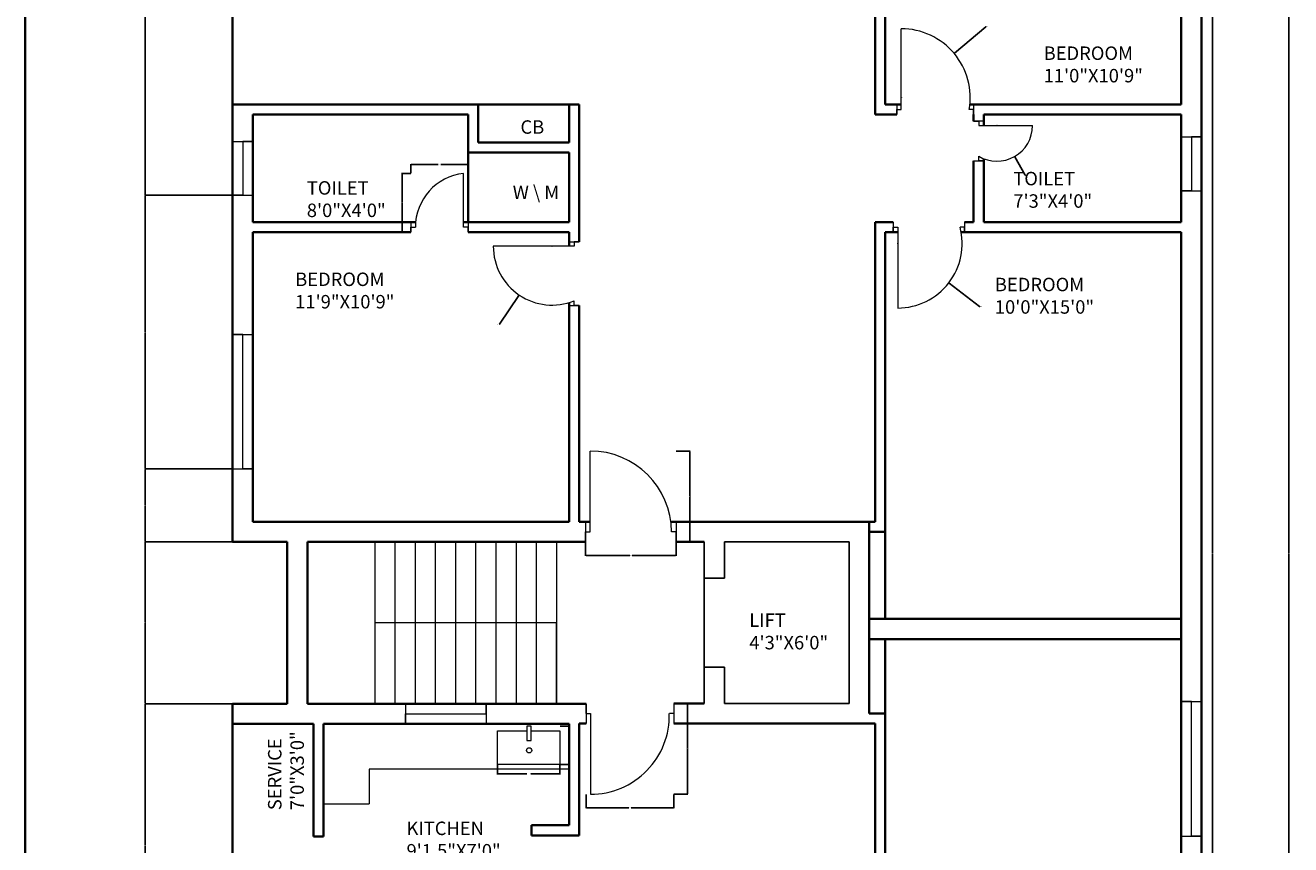
# Model space of a CAD drawing. Units: inches. Extents: x 2250 to 3547, y 1387 to 2604.
# Tile 2 of 11: x 2250 to 2814, y 1765 to 2130. Entities that reach past the tile are written whole.
import ezdxf

# ---------------------------------------------------------------- set-up
doc = ezdxf.new("R2010")
doc.units = ezdxf.units.IN
for name, color, linetype, lineweight in [('A-ANNO-DIMS', 2, 'Continuous', 18), ('A-ANNO-TTLB', 7, 'Continuous', 35), ('A-AREA-IDEN', 7, 'Continuous', 18), ('A-DOOR', 3, 'Continuous', 18), ('A-FLOR-CASE', 9, 'Continuous', 18), ('A-FLOR-EVTR', 6, 'Continuous', 25), ('A-FLOR-FIXT', 8, 'Continuous', 18), ('A-FLOR-STRS', 7, 'Continuous', 18), ('A-GLAZ', 4, 'Continuous', 18), ('A-WALL', 7, 'Continuous', 35)]:
    doc.layers.add(name, color=color, linetype=linetype, lineweight=lineweight)
doc.styles.get("Standard").update_dxf_attribs({"font": 'arial.ttf'})
doc.dimstyles.get("Standard").update_dxf_attribs({"dimtxt": 0.18, "dimasz": 0.18, "dimexe": 0.18, "dimexo": 0.0625, "dimgap": 0.09, "dimtad": 0, "dimtih": 1, "dimtoh": 1, "dimdec": 4, "dimzin": 0, "dimdsep": 46, "dimtxsty": 'Standard', "dimcen": 0.09, "dimadec": 0, "dimazin": 0, "dimtfac": 1, "dimtdec": 4, "dimtofl": 0, "dimtmove": 0, "dimatfit": 3, "dimfxl": 1, "dimtolj": 1, "dimtzin": 0, "dimarcsym": 0})

# ---------------------------------------------------------------- blocks, each defined once
blk = doc.blocks.new('WIN-24')
for p, q in [((0, 24), (9, 24)), ((9, 24), (4.5, 24)), ((4.5, 24), (4.5, 0)), ((4.5, 0), (0, 0)), ((0, 0), (9, 0))]:
    blk.add_line(p, q)
blk = doc.blocks.new('WIN-60')
for p, q in [((0, 9), (0, 0)), ((60, 4.5), (60, 9)), ((60, 9), (60, 0)), ((0, 0), (0, 4.5)), ((0, 4.5), (60, 4.5))]:
    blk.add_line(p, q)
blk = doc.blocks.new('WIN-36')
for p, q in [((0, 9), (0, 0)), ((36, 4.5), (36, 9)), ((36, 9), (36, 0)), ((0, 0), (0, 4.5)), ((0, 4.5), (36, 4.5))]:
    blk.add_line(p, q)
blk = doc.blocks.new('DOOR-BED-NORTHEAST')
for p, q in [((2, 2.25), (2, 38.25)), ((0, 4.5), (0, 0)), ((0, 0), (0, 2.25)), ((0, 2.25), (2, 2.25)), ((34.25, 2.25), (32.25, 2.25)), ((34.25, 4.5), (34.25, 0)), ((34.25, 0), (34.25, 2.25))]:
    blk.add_line(p, q)
blk.add_arc((2, 7.54), 30.71, 350.0755, 90)
blk = doc.blocks.new('DOOR-BED-WEST-N')
for p, q in [((33.75, 28.33), (38.25, 28.33)), ((38.25, 28.33), (36, 28.33)), ((36, 28.33), (36, 26.33)), ((36, 26.33), (0, 26.33)), ((33.75, 0), (38.25, 0)), ((36, 0), (36, 2)), ((38.25, 0), (36, 0))]:
    blk.add_line(p, q)
blk.add_arc((26.22, 26.33), 26.22, 180, 291.8953)
blk = doc.blocks.new('DOOR-BATH-WEST-N')
for p, q in [((23.5, 2.25), (23.5, 26.25)), ((0, 4.5), (0, 0)), ((0, 0), (0, 2.25)), ((0, 2.25), (2, 2.25)), ((25.5, 2.25), (23.5, 2.25)), ((25.5, 4.5), (25.5, 0)), ((25.5, 0), (25.5, 2.25))]:
    blk.add_line(p, q)
blk.add_arc((26.15, 2.25), 24.15, 96.2899, 180)
blk = doc.blocks.new('DOOR-BATH-EAST-N')
for p, q in [((4.5, 17.63), (0, 17.63)), ((0, 17.63), (2.25, 17.63)), ((2.25, 17.63), (2.25, 15.63)), ((2.25, 15.63), (26.25, 15.63)), ((0, 0), (4.5, 0)), ((2.25, 0), (2.25, 2)), ((4.5, 0), (2.25, 0))]:
    blk.add_line(p, q)
blk.add_arc((10.38, 15.63), 15.87, 239.2006, 0)
blk = doc.blocks.new('DOOR-BED-EAST-N')
for p, q in [((0, 38.25), (0, 33.75)), ((0, 33.75), (0, 36)), ((0, 36), (2, 36)), ((2, 36), (2, 0)), ((31.84, 36), (29.84, 36)), ((31.84, 38.25), (31.84, 33.75)), ((31.84, 33.75), (31.84, 36))]:
    blk.add_line(p, q)
blk.add_arc((2, 28.77), 28.77, 270, 14.5631)
blk = doc.blocks.new('DOOR-LOBBY-NORTH')
for p, q in [((2, 4.5), (2, 40.5)), ((0, 9), (0, 0)), ((40.31, 9), (40.31, 0)), ((0, 0), (0, 4.5)), ((0, 4.5), (2, 4.5)), ((40.31, 4.5), (38.31, 4.5)), ((40.31, 0), (40.31, 4.5))]:
    blk.add_line(p, q)
blk.add_arc((2, 4.19), 36.31, 0.4922, 90)
blk = doc.blocks.new('DOOR-LOBBY-SOUTH')
for p, q in [((0, 36), (0, 40.36)), ((0, 40.36), (0, 31.5)), ((39.15, 40.5), (39.15, 31.5)), ((0, 36), (2, 36)), ((2, 36), (2, 0)), ((39.15, 36), (37.15, 36))]:
    blk.add_line(p, q)
blk.add_arc((2, 35.16), 35.16, 270, 1.3721)
blk = doc.blocks.new('KITCHEN-SINK-SINGLE')
blk.add_lwpolyline([(14.98, 17.19), (13.12, 17.19), (13.12, 10.67), (14.98, 10.67)], close=True)
blk.add_lwpolyline([(14.98, 15.02), (27.83, 15.02), (27.83, 0), (0, 0), (0, 15.02), (13.12, 15.02)])
blk.add_circle((14.09, 6.33), 1.15)
blk = doc.blocks.new('STAIR-FLIGHT')
for p, q in [((0, 72.14), (0, 0)), ((9, 72.14), (9, 0)), ((18, 72.14), (18, 0)), ((27, 72.14), (27, 0)), ((36, 72.14), (36, 0)), ((45, 72.14), (45, 0)), ((54, 72.14), (54, 0)), ((63, 72.14), (63, 0)), ((72, 72.14), (72, 0)), ((81, 72.14), (81, 0)), ((81, 36.07), (0, 36.07)), ((81, 0), (81, 36.07))]:
    blk.add_line(p, q)
blk = doc.blocks.new('LIFT-SHAFT')
for p, q in [((0, 72), (0, 55.86)), ((9, 72), (60, 72)), ((9, 55.86), (9, 72)), ((60, 72), (64.53, 72)), ((64.53, 72), (64.53, 0)), ((0, 55.86), (9, 55.86)), ((0, 55.86), (0, 16.11)), ((0, 16.11), (9, 16.11)), ((0, 16.11), (0, 0)), ((9, 0), (9, 16.11)), ((60, 0), (9, 0)), ((9, 0), (60, 0)), ((64.53, 0), (60, 0))]:
    blk.add_line(p, q)
blk = doc.blocks.new('*D52')
at = {"layer": 'A-ANNO-DIMS', "color": 0, "lineweight": -2, "transparency": 16777216}
for p, q in [((2421.98, 2063.81), (2417.92, 2063.81)), ((2418.1, 2063.63), (2418.1, 2050.87)), ((2418.1, 2037.74), (2418.1, 2050.51)), ((2421.98, 2037.56), (2417.92, 2037.56))]:
    blk.add_line(p, q, dxfattribs=at)
at = {"layer": 'A-ANNO-DIMS', "color": 0, "transparency": 16777216}
for points in [[(2418.07, 2063.63), (2418.13, 2063.63), (2418.1, 2063.81)], [(2418.07, 2037.74), (2418.13, 2037.74), (2418.1, 2037.56)]]:
    blk.add_solid(points, dxfattribs=at)
at = {"layer": 'Defpoints', "color": 0, "transparency": 16777216}
for p in [(2418.1, 2063.81), (2422.04, 2063.81), (2422.04, 2037.56)]:
    blk.add_point(p, dxfattribs=at)
at = {"layer": 'A-ANNO-DIMS', "color": 0, "transparency": 16777216, "insert": (2418.1, 2050.69), "char_height": 0.18, "attachment_point": 5}
blk.add_mtext('\\A1;DOOR 26 TYP.', dxfattribs=at)
blk = doc.blocks.new('*D53')
at = {"layer": 'A-ANNO-DIMS', "color": 0, "lineweight": -2, "transparency": 16777216}
for p, q in [((2422.04, 2063.88), (2422.04, 2067.93)), ((2422.22, 2067.75), (2434.26, 2067.75)), ((2447.36, 2067.75), (2435.32, 2067.75)), ((2447.54, 2063.88), (2447.54, 2067.93))]:
    blk.add_line(p, q, dxfattribs=at)
at = {"layer": 'A-ANNO-DIMS', "color": 0, "transparency": 16777216}
for points in [[(2422.22, 2067.78), (2422.22, 2067.72), (2422.04, 2067.75)], [(2447.36, 2067.78), (2447.36, 2067.72), (2447.54, 2067.75)]]:
    blk.add_solid(points, dxfattribs=at)
at = {"layer": 'Defpoints', "color": 0, "transparency": 16777216}
for p in [(2447.54, 2067.75), (2422.04, 2063.81), (2447.54, 2063.81)]:
    blk.add_point(p, dxfattribs=at)
at = {"layer": 'A-ANNO-DIMS', "color": 0, "transparency": 16777216, "insert": (2434.79, 2067.75), "char_height": 0.18, "attachment_point": 5}
blk.add_mtext('\\A1;26 TYP.', dxfattribs=at)
blk = doc.blocks.new('*D60')
at = {"layer": 'A-ANNO-DIMS', "color": 0, "lineweight": -2, "transparency": 16777216}
for p, q in [((2540.34, 1940.06), (2546.53, 1940.06)), ((2546.35, 1939.88), (2546.35, 1920)), ((2546.35, 1899.74), (2546.35, 1919.63)), ((2540.34, 1899.56), (2546.53, 1899.56))]:
    blk.add_line(p, q, dxfattribs=at)
at = {"layer": 'A-ANNO-DIMS', "color": 0, "transparency": 16777216}
for points in [[(2546.32, 1939.88), (2546.38, 1939.88), (2546.35, 1940.06)], [(2546.32, 1899.74), (2546.38, 1899.74), (2546.35, 1899.56)]]:
    blk.add_solid(points, dxfattribs=at)
at = {"layer": 'Defpoints', "color": 0, "transparency": 16777216}
for p in [(2540.27, 1940.06), (2546.35, 1940.06), (2540.27, 1899.56)]:
    blk.add_point(p, dxfattribs=at)
at = {"layer": 'A-ANNO-DIMS', "color": 0, "transparency": 16777216, "insert": (2546.35, 1919.81), "char_height": 0.18, "attachment_point": 5}
blk.add_mtext('\\A1;DOOR 41 TYP.', dxfattribs=at)
blk = doc.blocks.new('*D61')
at = {"layer": 'A-ANNO-DIMS', "color": 0, "lineweight": -2, "transparency": 16777216}
for p, q in [((2499.96, 1899.5), (2499.96, 1893.31)), ((2540.27, 1899.5), (2540.27, 1893.31)), ((2500.14, 1893.49), (2519.59, 1893.49)), ((2540.09, 1893.49), (2520.65, 1893.49))]:
    blk.add_line(p, q, dxfattribs=at)
at = {"layer": 'A-ANNO-DIMS', "color": 0, "transparency": 16777216}
for points in [[(2500.14, 1893.52), (2500.14, 1893.46), (2499.96, 1893.49)], [(2540.09, 1893.52), (2540.09, 1893.46), (2540.27, 1893.49)]]:
    blk.add_solid(points, dxfattribs=at)
at = {"layer": 'Defpoints', "color": 0, "transparency": 16777216}
for p in [(2499.96, 1899.56), (2540.27, 1899.56), (2540.27, 1893.49)]:
    blk.add_point(p, dxfattribs=at)
at = {"layer": 'A-ANNO-DIMS', "color": 0, "transparency": 16777216, "insert": (2520.12, 1893.49), "char_height": 0.18, "attachment_point": 5}
blk.add_mtext('\\A1;40 TYP.', dxfattribs=at)
blk = doc.blocks.new('*D64')
at = {"layer": 'A-ANNO-DIMS', "color": 0, "lineweight": -2, "transparency": 16777216}
for p, q in [((2539.33, 1827.56), (2545.53, 1827.56)), ((2545.35, 1827.38), (2545.35, 1807.5)), ((2545.35, 1787.24), (2545.35, 1807.13)), ((2539.33, 1787.06), (2545.53, 1787.06))]:
    blk.add_line(p, q, dxfattribs=at)
at = {"layer": 'A-ANNO-DIMS', "color": 0, "transparency": 16777216}
for points in [[(2545.32, 1827.38), (2545.38, 1827.38), (2545.35, 1827.56)], [(2545.32, 1787.24), (2545.38, 1787.24), (2545.35, 1787.06)]]:
    blk.add_solid(points, dxfattribs=at)
at = {"layer": 'Defpoints', "color": 0, "transparency": 16777216}
for p in [(2539.27, 1827.56), (2545.35, 1827.56), (2539.27, 1787.06)]:
    blk.add_point(p, dxfattribs=at)
at = {"layer": 'A-ANNO-DIMS', "color": 0, "transparency": 16777216, "insert": (2545.35, 1807.31), "char_height": 0.18, "attachment_point": 5}
blk.add_mtext('\\A1;DOOR 41 TYP.', dxfattribs=at)
blk = doc.blocks.new('*D65')
at = {"layer": 'A-ANNO-DIMS', "color": 0, "lineweight": -2, "transparency": 16777216}
for p, q in [((2500.12, 1787), (2500.12, 1780.81)), ((2539.27, 1787), (2539.27, 1780.81)), ((2500.3, 1780.99), (2519.17, 1780.99)), ((2539.09, 1780.99), (2520.23, 1780.99))]:
    blk.add_line(p, q, dxfattribs=at)
at = {"layer": 'A-ANNO-DIMS', "color": 0, "transparency": 16777216}
for points in [[(2500.3, 1781.02), (2500.3, 1780.96), (2500.12, 1780.99)], [(2539.09, 1781.02), (2539.09, 1780.96), (2539.27, 1780.99)]]:
    blk.add_solid(points, dxfattribs=at)
at = {"layer": 'Defpoints', "color": 0, "transparency": 16777216}
for p in [(2500.12, 1787.06), (2539.27, 1787.06), (2539.27, 1780.99)]:
    blk.add_point(p, dxfattribs=at)
at = {"layer": 'A-ANNO-DIMS', "color": 0, "transparency": 16777216, "insert": (2519.7, 1780.99), "char_height": 0.18, "attachment_point": 5}
blk.add_mtext('\\A1;39 TYP.', dxfattribs=at)
blk = doc.blocks.new('*D68')
at = {"layer": 'A-ANNO-DIMS', "color": 0, "lineweight": -2, "transparency": 16777216}
for p, q in [((2460.68, 1800.23), (2460.68, 1795.94)), ((2488.5, 1800.23), (2488.5, 1795.94)), ((2460.86, 1796.12), (2473.73, 1796.12)), ((2488.32, 1796.12), (2475.45, 1796.12))]:
    blk.add_line(p, q, dxfattribs=at)
at = {"layer": 'A-ANNO-DIMS', "color": 0, "transparency": 16777216}
for points in [[(2460.86, 1796.15), (2460.86, 1796.09), (2460.68, 1796.12)], [(2488.32, 1796.15), (2488.32, 1796.09), (2488.5, 1796.12)]]:
    blk.add_solid(points, dxfattribs=at)
at = {"layer": 'Defpoints', "color": 0, "transparency": 16777216}
for p in [(2460.68, 1800.29), (2488.5, 1800.29), (2488.5, 1796.12)]:
    blk.add_point(p, dxfattribs=at)
at = {"layer": 'A-ANNO-DIMS', "color": 0, "transparency": 16777216, "insert": (2474.59, 1796.12), "char_height": 0.18, "attachment_point": 5}
blk.add_mtext('\\A1;SINK 28 TYP.', dxfattribs=at)
blk = doc.blocks.new('*D69')
at = {"layer": 'A-ANNO-DIMS', "color": 0, "lineweight": -2, "transparency": 16777216}
for p, q in [((2488.57, 1817.48), (2492.86, 1817.48)), ((2492.68, 1817.3), (2492.68, 1809.07)), ((2492.68, 1800.47), (2492.68, 1808.71)), ((2488.57, 1800.29), (2492.86, 1800.29))]:
    blk.add_line(p, q, dxfattribs=at)
at = {"layer": 'A-ANNO-DIMS', "color": 0, "transparency": 16777216}
for points in [[(2492.65, 1817.3), (2492.71, 1817.3), (2492.68, 1817.48)], [(2492.65, 1800.47), (2492.71, 1800.47), (2492.68, 1800.29)]]:
    blk.add_solid(points, dxfattribs=at)
at = {"layer": 'Defpoints', "color": 0, "transparency": 16777216}
for p in [(2488.5, 1817.48), (2492.68, 1817.48), (2488.5, 1800.29)]:
    blk.add_point(p, dxfattribs=at)
at = {"layer": 'A-ANNO-DIMS', "color": 0, "transparency": 16777216, "insert": (2492.68, 1808.89), "char_height": 0.18, "attachment_point": 5}
blk.add_mtext('\\A1;17 TYP.', dxfattribs=at)
blk = doc.blocks.new('*D77')
at = {"layer": 'A-ANNO-DIMS', "color": 0, "lineweight": -2, "transparency": 16777216}
for p, q in [((2633.6, 2245.18), (2813.67, 2245.18)), ((2813.49, 2245), (2813.49, 1894.73)), ((2813.49, 1544.1), (2813.49, 1894.37)), ((2774.6, 1543.92), (2813.67, 1543.92))]:
    blk.add_line(p, q, dxfattribs=at)
at = {"layer": 'A-ANNO-DIMS', "color": 0, "transparency": 16777216}
for points in [[(2813.46, 2245), (2813.52, 2245), (2813.49, 2245.18)], [(2813.46, 1544.1), (2813.52, 1544.1), (2813.49, 1543.92)]]:
    blk.add_solid(points, dxfattribs=at)
at = {"layer": 'Defpoints', "color": 0, "transparency": 16777216}
for p in [(2633.54, 2245.18), (2813.49, 2245.18), (2774.54, 1543.92)]:
    blk.add_point(p, dxfattribs=at)
at = {"layer": 'A-ANNO-DIMS', "color": 0, "transparency": 16777216, "insert": (2813.49, 1894.55), "char_height": 0.18, "attachment_point": 5}
blk.add_mtext('\\A1;701.3', dxfattribs=at)
blk = doc.blocks.new('*D79')
at = {"layer": 'A-ANNO-DIMS', "color": 0, "lineweight": -2, "transparency": 16777216}
for p, q in [((2342.48, 1827.42), (2303.41, 1827.42)), ((2303.59, 1827.24), (2303.59, 1764.55)), ((2303.59, 1701.5), (2303.59, 1764.19)), ((2342.48, 1701.32), (2303.41, 1701.32))]:
    blk.add_line(p, q, dxfattribs=at)
at = {"layer": 'A-ANNO-DIMS', "color": 0, "transparency": 16777216}
for points in [[(2303.56, 1827.24), (2303.62, 1827.24), (2303.59, 1827.42)], [(2303.56, 1701.5), (2303.62, 1701.5), (2303.59, 1701.32)]]:
    blk.add_solid(points, dxfattribs=at)
at = {"layer": 'Defpoints', "color": 0, "transparency": 16777216}
for p in [(2303.59, 1827.42), (2342.54, 1827.42), (2342.54, 1701.32)]:
    blk.add_point(p, dxfattribs=at)
at = {"layer": 'A-ANNO-DIMS', "color": 0, "transparency": 16777216, "insert": (2303.59, 1764.37), "char_height": 0.18, "attachment_point": 5}
blk.add_mtext('\\A1;126.1', dxfattribs=at)
blk = doc.blocks.new('*D80')
at = {"layer": 'A-ANNO-DIMS', "color": 0, "lineweight": -2, "transparency": 16777216}
for p, q in [((2342.48, 1899.56), (2303.41, 1899.56)), ((2303.59, 1899.38), (2303.59, 1863.67)), ((2303.59, 1827.6), (2303.59, 1863.31)), ((2342.48, 1827.42), (2303.41, 1827.42))]:
    blk.add_line(p, q, dxfattribs=at)
at = {"layer": 'A-ANNO-DIMS', "color": 0, "transparency": 16777216}
for points in [[(2303.56, 1899.38), (2303.62, 1899.38), (2303.59, 1899.56)], [(2303.56, 1827.6), (2303.62, 1827.6), (2303.59, 1827.42)]]:
    blk.add_solid(points, dxfattribs=at)
at = {"layer": 'Defpoints', "color": 0, "transparency": 16777216}
for p in [(2303.59, 1899.56), (2342.54, 1899.56), (2342.54, 1827.42)]:
    blk.add_point(p, dxfattribs=at)
at = {"layer": 'A-ANNO-DIMS', "color": 0, "transparency": 16777216, "insert": (2303.59, 1863.49), "char_height": 0.18, "attachment_point": 5}
blk.add_mtext('\\A1;72.14', dxfattribs=at)
blk = doc.blocks.new('*D81')
at = {"layer": 'A-ANNO-DIMS', "color": 0, "lineweight": -2, "transparency": 16777216}
for p, q in [((2342.48, 1932.06), (2303.41, 1932.06)), ((2303.59, 1931.88), (2303.59, 1915.99)), ((2303.59, 1899.74), (2303.59, 1915.63)), ((2342.48, 1899.56), (2303.41, 1899.56))]:
    blk.add_line(p, q, dxfattribs=at)
at = {"layer": 'A-ANNO-DIMS', "color": 0, "transparency": 16777216}
for points in [[(2303.56, 1931.88), (2303.62, 1931.88), (2303.59, 1932.06)], [(2303.56, 1899.74), (2303.62, 1899.74), (2303.59, 1899.56)]]:
    blk.add_solid(points, dxfattribs=at)
at = {"layer": 'Defpoints', "color": 0, "transparency": 16777216}
for p in [(2303.59, 1932.06), (2342.54, 1932.06), (2342.54, 1899.56)]:
    blk.add_point(p, dxfattribs=at)
at = {"layer": 'A-ANNO-DIMS', "color": 0, "transparency": 16777216, "insert": (2303.59, 1915.81), "char_height": 0.18, "attachment_point": 5}
blk.add_mtext('\\A1;32.494', dxfattribs=at)
blk = doc.blocks.new('*D82')
at = {"layer": 'A-ANNO-DIMS', "color": 0, "lineweight": -2, "transparency": 16777216}
for p, q in [((2342.48, 2054.09), (2303.41, 2054.09)), ((2303.59, 2053.91), (2303.59, 1993.26)), ((2303.59, 1932.24), (2303.59, 1992.89)), ((2342.48, 1932.06), (2303.41, 1932.06))]:
    blk.add_line(p, q, dxfattribs=at)
at = {"layer": 'A-ANNO-DIMS', "color": 0, "transparency": 16777216}
for points in [[(2303.56, 2053.91), (2303.62, 2053.91), (2303.59, 2054.09)], [(2303.56, 1932.24), (2303.62, 1932.24), (2303.59, 1932.06)]]:
    blk.add_solid(points, dxfattribs=at)
at = {"layer": 'Defpoints', "color": 0, "transparency": 16777216}
for p in [(2303.59, 2054.09), (2342.54, 2054.09), (2342.54, 1932.06)]:
    blk.add_point(p, dxfattribs=at)
at = {"layer": 'A-ANNO-DIMS', "color": 0, "transparency": 16777216, "insert": (2303.59, 1993.07), "char_height": 0.18, "attachment_point": 5}
blk.add_mtext('\\A1;122.03', dxfattribs=at)
blk = doc.blocks.new('*D83')
at = {"layer": 'A-ANNO-DIMS', "color": 0, "lineweight": -2, "transparency": 16777216}
for p, q in [((2342.48, 2232.56), (2303.41, 2232.56)), ((2303.59, 2232.38), (2303.59, 2143.51)), ((2303.59, 2054.27), (2303.59, 2143.15)), ((2342.48, 2054.09), (2303.41, 2054.09))]:
    blk.add_line(p, q, dxfattribs=at)
at = {"layer": 'A-ANNO-DIMS', "color": 0, "transparency": 16777216}
for points in [[(2303.56, 2232.38), (2303.62, 2232.38), (2303.59, 2232.56)], [(2303.56, 2054.27), (2303.62, 2054.27), (2303.59, 2054.09)]]:
    blk.add_solid(points, dxfattribs=at)
at = {"layer": 'Defpoints', "color": 0, "transparency": 16777216}
for p in [(2303.59, 2232.56), (2342.54, 2232.56), (2342.54, 2054.09)]:
    blk.add_point(p, dxfattribs=at)
at = {"layer": 'A-ANNO-DIMS', "color": 0, "transparency": 16777216, "insert": (2303.59, 2143.33), "char_height": 0.18, "attachment_point": 5}
blk.add_mtext('\\A1;178.47', dxfattribs=at)
blk = doc.blocks.new('*D85')
at = {"layer": 'A-ANNO-DIMS', "color": 0, "lineweight": -2, "transparency": 16777216}
for p, q in [((3001.57, 2245.18), (2779.34, 2245.18)), ((2779.52, 2245), (2779.52, 1894.73)), ((2779.52, 1544.1), (2779.52, 1894.37)), ((2851.57, 1543.92), (2779.34, 1543.92))]:
    blk.add_line(p, q, dxfattribs=at)
at = {"layer": 'A-ANNO-DIMS', "color": 0, "transparency": 16777216}
for points in [[(2779.49, 2245), (2779.55, 2245), (2779.52, 2245.18)], [(2779.49, 1544.1), (2779.55, 1544.1), (2779.52, 1543.92)]]:
    blk.add_solid(points, dxfattribs=at)
at = {"layer": 'Defpoints', "color": 0, "transparency": 16777216}
for p in [(2779.52, 2245.18), (3001.63, 2245.18), (2851.63, 1543.92)]:
    blk.add_point(p, dxfattribs=at)
at = {"layer": 'A-ANNO-DIMS', "color": 0, "transparency": 16777216, "insert": (2779.52, 1894.55), "char_height": 0.18, "attachment_point": 5}
blk.add_mtext('\\A1;701.3', dxfattribs=at)
blk = doc.blocks.new('*D117')
at = {"layer": 'A-ANNO-DIMS', "color": 0, "lineweight": -2, "transparency": 16777216}
for p, q in [((2678.33, 2129.21), (2664.36, 2117.48)), ((2678.51, 2129.21), (2678.33, 2129.21)), ((2640.63, 2097.61), (2640.81, 2097.61)), ((2640.72, 2097.52), (2640.72, 2097.7))]:
    blk.add_line(p, q, dxfattribs=at)
at = {"layer": 'A-ANNO-DIMS', "color": 0, "transparency": 16777216}
blk.add_solid([(2664.34, 2117.5), (2664.38, 2117.45), (2664.23, 2117.36)], dxfattribs=at)
at = {"layer": 'Defpoints', "color": 0, "transparency": 16777216}
for p in [(2664.23, 2117.36), (2640.72, 2097.61)]:
    blk.add_point(p, dxfattribs=at)
at = {"layer": 'A-ANNO-DIMS', "color": 0, "transparency": 16777216, "insert": (2678.97, 2129.21), "char_height": 0.18, "attachment_point": 5}
blk.add_mtext('\\A1;R30.71', dxfattribs=at)
blk = doc.blocks.new('*D119')
at = {"layer": 'A-ANNO-DIMS', "color": 0, "lineweight": -2, "transparency": 16777216}
for p, q in [((2639, 2032.58), (2639.18, 2032.58)), ((2639.09, 2032.49), (2639.09, 2032.67)), ((2675.5, 2004.42), (2661.98, 2014.87)), ((2675.68, 2004.42), (2675.5, 2004.42))]:
    blk.add_line(p, q, dxfattribs=at)
at = {"layer": 'A-ANNO-DIMS', "color": 0, "transparency": 16777216}
blk.add_solid([(2662, 2014.9), (2661.97, 2014.85), (2661.84, 2014.98)], dxfattribs=at)
at = {"layer": 'Defpoints', "color": 0, "transparency": 16777216}
for p in [(2639.09, 2032.58), (2661.84, 2014.98)]:
    blk.add_point(p, dxfattribs=at)
at = {"layer": 'A-ANNO-DIMS', "color": 0, "transparency": 16777216, "insert": (2676.23, 2004.42), "char_height": 0.18, "attachment_point": 5}
blk.add_mtext('\\A1;R28.767', dxfattribs=at)
blk = doc.blocks.new('*D122')
at = {"layer": 'A-ANNO-DIMS', "color": 0, "lineweight": -2, "transparency": 16777216}
for p, q in [((2484.92, 2031.32), (2485.1, 2031.32)), ((2485.01, 2031.23), (2485.01, 2031.41)), ((2461.52, 1996.56), (2470.23, 2009.45)), ((2461.34, 1996.56), (2461.52, 1996.56))]:
    blk.add_line(p, q, dxfattribs=at)
at = {"layer": 'A-ANNO-DIMS', "color": 0, "transparency": 16777216}
blk.add_solid([(2470.2, 2009.46), (2470.25, 2009.43), (2470.33, 2009.6)], dxfattribs=at)
at = {"layer": 'Defpoints', "color": 0, "transparency": 16777216}
for p in [(2485.01, 2031.32), (2470.33, 2009.6)]:
    blk.add_point(p, dxfattribs=at)
at = {"layer": 'A-ANNO-DIMS', "color": 0, "transparency": 16777216, "insert": (2460.86, 1996.56), "char_height": 0.18, "attachment_point": 5}
blk.add_mtext('\\A1;R26.22', dxfattribs=at)
blk = doc.blocks.new('*D129')
at = {"layer": 'A-ANNO-DIMS', "color": 0, "lineweight": -2, "transparency": 16777216}
for p, q in [((2683.25, 2085.12), (2683.43, 2085.12)), ((2683.34, 2085.03), (2683.34, 2085.21)), ((2695.89, 2063.04), (2691.27, 2071.16)), ((2696.07, 2063.04), (2695.89, 2063.04))]:
    blk.add_line(p, q, dxfattribs=at)
at = {"layer": 'A-ANNO-DIMS', "color": 0, "transparency": 16777216}
blk.add_solid([(2691.3, 2071.18), (2691.24, 2071.15), (2691.18, 2071.32)], dxfattribs=at)
at = {"layer": 'Defpoints', "color": 0, "transparency": 16777216}
for p in [(2683.34, 2085.12), (2691.18, 2071.32)]:
    blk.add_point(p, dxfattribs=at)
at = {"layer": 'A-ANNO-DIMS', "color": 0, "transparency": 16777216, "insert": (2696.62, 2063.04), "char_height": 0.18, "attachment_point": 5}
blk.add_mtext('\\A1;R15.873', dxfattribs=at)

msp = doc.modelspace()

# ---------------------------------------------------------------- linework, layer by layer
at = {"layer": 'A-ANNO-TTLB'}
msp.add_lwpolyline([(2250.1093, 2604.1988), (3546.995, 2604.1988), (3546.995, 1386.7251), (2250.1093, 1386.7251)], close=True, dxfattribs=at)
at = {"layer": 'A-FLOR-CASE'}
for p, q in [((2492.5378, 1798.2531), (2403.4298, 1798.2531)), ((2403.4298, 1798.2531), (2403.4298, 1782.7382)), ((2383.0378, 1782.7382), (2403.4298, 1782.7382))]:
    msp.add_line(p, q, dxfattribs=at)
at = {"layer": 'A-WALL'}
for p, q in [((2342.5378, 2232.5639), (2342.5378, 1899.5639)), ((2342.5378, 2232.5639), (2342.5378, 1899.5639)), ((2774.5378, 2232.5639), (2774.5378, 1543.9245)), ((2633.5378, 2223.5639), (2633.5378, 2094.5639)), ((2765.5378, 2223.5639), (2765.5378, 2094.5639)), ((2629.0378, 2198.6762), (2629.0378, 2090.0639)), ((2342.5378, 2094.5639), (2452.0378, 2094.5639)), ((2452.0378, 2077.6358), (2452.0378, 2094.5639)), ((2492.5378, 2094.5639), (2452.0378, 2094.5639)), ((2492.5378, 2094.5639), (2492.5378, 2077.6358)), ((2492.5378, 2094.5639), (2497.0378, 2094.5639)), ((2497.0378, 2094.5639), (2497.0378, 2033.3217)), ((2633.5378, 2094.5639), (2640.7159, 2094.5639)), ((2671.2723, 2094.5639), (2765.5378, 2094.5639)), ((2351.5378, 2090.0639), (2447.5378, 2090.0639)), ((2351.5378, 2090.0639), (2351.5378, 2042.0639)), ((2351.5378, 2090.0639), (2447.5378, 2090.0639)), ((2447.5378, 2090.0639), (2447.5378, 2042.0639)), ((2629.0378, 2090.0639), (2638.7159, 2090.0639)), ((2672.9639, 2090.0639), (2672.9639, 2087.1197)), ((2677.4639, 2090.0639), (2765.5378, 2090.0639)), ((2677.4639, 2090.0639), (2677.4639, 2087.1197)), ((2677.4639, 2085.1197), (2677.4639, 2090.0639)), ((2765.5378, 2090.0639), (2765.5378, 2042.0639)), ((2492.5378, 2077.6358), (2452.0378, 2077.6358)), ((2447.5378, 2073.1358), (2492.5378, 2073.1358)), ((2492.5378, 2073.1358), (2492.5378, 2042.0639)), ((2672.9639, 2069.4856), (2672.9639, 2042.0639)), ((2677.4639, 2042.0639), (2677.4639, 2070.3753)), ((2351.5378, 2042.0639), (2424.1429, 2042.0639)), ((2351.5378, 2037.5639), (2422.0378, 2037.5639)), ((2351.5378, 2037.5639), (2351.5378, 1908.5639)), ((2351.5378, 2037.5639), (2351.5378, 1908.5639)), ((2445.5378, 2042.0639), (2492.5378, 2042.0639)), ((2447.5378, 2037.5639), (2492.5378, 2037.5639)), ((2492.5378, 2037.5639), (2492.5378, 2031.3217)), ((2629.0378, 2042.0639), (2629.0378, 1908.5639)), ((2637.0867, 2042.0639), (2629.0378, 2042.0639)), ((2633.5378, 2037.5639), (2633.5378, 1908.5639)), ((2639.0867, 2037.5639), (2633.5378, 2037.5639)), ((2672.9639, 2037.5639), (2667.4185, 2037.5639)), ((2672.9639, 2042.0639), (2668.9291, 2042.0639)), ((2672.9639, 2037.5639), (2765.5378, 2037.5639)), ((2672.9639, 2037.5639), (2677.4639, 2037.5639)), ((2677.4639, 2042.0639), (2765.5378, 2042.0639)), ((2765.5378, 2037.5639), (2765.5378, 1727.1967)), ((2492.5378, 2006.204), (2492.5378, 1908.5639)), ((2497.0378, 2004.9915), (2497.0378, 1908.5639)), ((2351.5378, 1908.5639), (2492.5378, 1908.5639)), ((2497.0378, 1908.5639), (2501.9628, 1908.5639)), ((2537.9545, 1908.5639), (2629.0378, 1908.5639)), ((2617.3962, 1908.5639), (2626.3962, 1908.5639)), ((2626.3962, 1908.5639), (2626.3962, 1823.0639)), ((2626.3962, 1908.5639), (2626.3962, 1904.0639)), ((2633.5378, 1908.5639), (2633.5378, 1865.1967)), ((2626.3962, 1904.0639), (2633.5378, 1904.0639)), ((2366.9248, 1899.5639), (2342.5378, 1899.5639)), ((2366.9248, 1899.5639), (2366.9248, 1827.4245)), ((2492.5378, 1899.5639), (2375.9248, 1899.5639)), ((2375.9248, 1827.4245), (2375.9248, 1899.5639)), ((2492.5378, 1899.5639), (2497.0378, 1899.5639)), ((2497.0378, 1899.5639), (2499.9628, 1899.5639)), ((2540.2734, 1899.5639), (2552.8654, 1899.5639)), ((2626.3962, 1865.1967), (2765.5378, 1865.1967)), ((2765.5378, 1865.1967), (2765.5378, 1856.1967)), ((2765.5378, 1856.1967), (2626.3962, 1856.1967)), ((2633.5378, 1856.1967), (2633.5378, 1727.1967)), ((2342.5378, 1827.4245), (2342.5378, 1543.9245)), ((2342.5378, 1827.4245), (2342.5378, 1543.9245)), ((2342.5378, 1827.4245), (2342.5378, 1818.4245)), ((2366.9248, 1827.4245), (2342.5378, 1827.4245)), ((2500.1234, 1827.4245), (2375.9248, 1827.4245)), ((2539.2714, 1827.5639), (2552.8654, 1827.5639)), ((2626.3962, 1823.0639), (2633.5378, 1823.0639)), ((2342.5378, 1818.4245), (2378.5378, 1818.4245)), ((2378.5378, 1818.4245), (2378.5378, 1768.2118)), ((2383.0378, 1818.4245), (2383.0378, 1768.2118)), ((2383.0378, 1818.4245), (2492.5378, 1818.4245)), ((2492.5378, 1818.4245), (2492.5378, 1773.2235)), ((2497.0378, 1818.5639), (2500.1234, 1818.5639)), ((2497.0378, 1818.5639), (2497.0378, 1768.7235)), ((2539.2714, 1818.5639), (2629.0378, 1818.5639)), ((2629.0378, 1818.5639), (2629.0378, 1722.6967)), ((2475.8174, 1768.7235), (2475.8174, 1773.2235)), ((2475.8174, 1773.2235), (2492.5378, 1773.2235)), ((2378.5378, 1768.2118), (2383.0378, 1768.2118)), ((2497.0378, 1768.7235), (2475.8174, 1768.7235)), ((2492.5378, 1768.7235), (2497.0378, 1768.7235))]:
    msp.add_line(p, q, dxfattribs=at)

# ---------------------------------------------------------------- block references
at = {"layer": 'A-DOOR'}
for name, p in [('DOOR-BED-NORTHEAST', (2638.7159, 2090.0639)), ('DOOR-BATH-EAST-N', (2672.9639, 2069.4856)), ('DOOR-BATH-WEST-N', (2422.0378, 2037.5639)), ('DOOR-BED-EAST-N', (2637.0867, 2003.8139)), ('DOOR-BED-WEST-N', (2458.7878, 2004.9915)), ('DOOR-LOBBY-NORTH', (2499.9628, 1899.5639)), ('DOOR-LOBBY-SOUTH', (2500.1234, 1787.0639))]:
    msp.add_blockref(name, p, dxfattribs=at)
at = {"layer": 'A-FLOR-EVTR'}
msp.add_blockref('LIFT-SHAFT', (2552.8654, 1827.5639), dxfattribs=at)
at = {"layer": 'A-FLOR-FIXT'}
msp.add_blockref('KITCHEN-SINK-SINGLE', (2460.6775, 1800.2946), dxfattribs=at)
at = {"layer": 'A-FLOR-STRS'}
msp.add_blockref('STAIR-FLIGHT', (2405.9149, 1827.4245), dxfattribs=at)
at = {"layer": 'A-GLAZ'}
for name, p in [('WIN-24', (2342.5378, 2054.091)), ('WIN-24', (2765.5378, 2056.0503)), ('WIN-36', (2419.5898, 1818.4245))]:
    msp.add_blockref(name, p, dxfattribs=at)
for p, rotation in [((2351.5378, 1932.0574), 90.00000000000158), ((2774.5378, 1768.424), 90.0000000000006)]:
    msp.add_blockref('WIN-60', p, dxfattribs=dict(at, rotation=rotation))

# ---------------------------------------------------------------- texts
at = {"layer": 'A-AREA-IDEN', "char_height": 6, "attachment_point": 1}
for s, width, insert in [('BEDROOM\\P11\'0"X10\'9"', 112.85603, (2704.1788, 2120.4041)), ('CB', 44.566869, (2470.8904, 2087.4932)), ('TOILET\\P8\'0"X4\'0"', 78.851075, (2375.6304, 2060.3582)), ('TOILET\\P7\'3"X4\'0"', 113.117025, (2690.6454, 2064.5094)), ('W \\\\ M', 51.713207, (2467.457, 2058.3963)), ('BEDROOM\\P11\'9"X10\'9"', 195.684104, (2370.4486, 2019.6184)), ('BEDROOM\\P10\'0"X15\'0"', 193.965785, (2682.4193, 2017.2862)), ('LIFT\\P4\'3"X6\'0"', 74.306581, (2572.928, 1867.649)), ('KITCHEN\\P9\'1.5"X7\'0"', 97.961769, (2420.0878, 1774.8651))]:
    msp.add_mtext_dynamic_manual_height_columns(s, width=width, gutter_width=12.5, heights=[0], dxfattribs=dict(at, insert=insert))
at = {"layer": 'A-AREA-IDEN', "insert": (2358.3355, 1779.9572), "char_height": 6, "attachment_point": 1, "rotation": 90}
msp.add_mtext_dynamic_manual_height_columns('SERVICE \\P7\'0"X3\'0"', width=317.1373, gutter_width=12.5, heights=[0], dxfattribs=at)

# ---------------------------------------------------------------- dimensions: what is measured, and where the dimension line sits
at = {"layer": 'A-ANNO-DIMS'}
for base, p1, p2, override, picture, middle in [((2813.4878, 2245.1762), (2774.5378, 1543.9245), (2633.5378, 2245.1762), {"dimdec": 1, "dimlfac": 1, "dimrnd": 0, "dimzin": 0, "dimdsep": 46, "dimlunit": 2}, '*D77', (2813.4878, 1894.5504)), ((2779.5165, 2245.1762), (2851.6288, 1543.9245), (3001.6288, 2245.1762), {"dimdec": 1, "dimlfac": 1, "dimrnd": 0, "dimzin": 0, "dimdsep": 46, "dimlunit": 2}, '*D85', (2779.5165, 1894.5504)), ((2303.5878, 2232.5639), (2342.5378, 2054.091), (2342.5378, 2232.5639), {"dimdec": 2, "dimlfac": 1, "dimrnd": 0, "dimzin": 0, "dimdsep": 46, "dimlunit": 2}, '*D83', (2303.5878, 2143.3274)), ((2303.5878, 2054.091), (2342.5378, 1932.0574), (2342.5378, 2054.091), {"dimdec": 2, "dimlfac": 1, "dimrnd": 0, "dimzin": 0, "dimdsep": 46, "dimlunit": 2}, '*D82', (2303.5878, 1993.0742)), ((2303.58781, 1932.05745), (2342.53781, 1899.56391), (2342.53781, 1932.05745), {"dimdec": 3, "dimlfac": 1, "dimrnd": 0, "dimzin": 0, "dimdsep": 46, "dimlunit": 2}, '*D81', (2303.58781, 1915.81068)), ((2303.5878, 1899.5639), (2342.5378, 1827.4245), (2342.5378, 1899.5639), {"dimdec": 2, "dimlfac": 1, "dimrnd": 0, "dimzin": 0, "dimdsep": 46, "dimlunit": 2}, '*D80', (2303.5878, 1863.4942)), ((2303.5878, 1827.4245), (2342.5378, 1701.3211), (2342.5378, 1827.4245), {"dimdec": 1, "dimlfac": 1, "dimrnd": 0, "dimzin": 0, "dimdsep": 46, "dimlunit": 2}, '*D79', (2303.5878, 1764.3728))]:
    dim = msp.add_linear_dim(base=base, p1=p1, p2=p2, angle=90, dimstyle='Standard', override=override, dxfattribs=at)
    dim.commit()
    dim.dimension.update_dxf_attribs({"geometry": picture, "text_midpoint": middle})
for center, mpoint, override, picture, middle in [((2640.7159, 2097.6064), (2664.2263, 2117.3602), {"dimdec": 2, "dimlfac": 1, "dimrnd": 0, "dimzin": 0, "dimdsep": 46, "dimlunit": 2}, '*D117', (2678.9749, 2129.2125)), ((2683.3412, 2085.1197), (2691.1813, 2071.3185), {"dimdec": 3, "dimlfac": 1, "dimrnd": 0, "dimzin": 0, "dimdsep": 46, "dimlunit": 2}, '*D129', (2696.6151, 2063.0377)), ((2485.0095, 2031.3217), (2470.3271, 2009.5961), {"dimdec": 2, "dimlfac": 1, "dimrnd": 0, "dimzin": 0, "dimdsep": 46, "dimlunit": 2}, '*D122', (2460.8587, 1996.5607)), ((2639.0867, 2032.5806), (2661.8421, 2014.9819), {"dimdec": 3, "dimlfac": 1, "dimrnd": 0, "dimzin": 0, "dimdsep": 46, "dimlunit": 2}, '*D119', (2676.2251, 2004.4227))]:
    dim = msp.add_radius_dim(center=center, mpoint=mpoint, dimstyle='Standard', override=override, dxfattribs=at)
    dim.commit()
    dim.dimension.update_dxf_attribs({"geometry": picture, "text_midpoint": middle, "dimtype": 164})
for base, p1, p2, text, picture, middle in [((2447.5378116389, 2067.7514100184), (2422.0378116389, 2063.8139100184), (2447.5378116389, 2063.8139100184), '<> TYP.', '*D53', (2434.7878116389, 2067.7514100184)), ((2540.2734, 1893.4889), (2499.9628, 1899.5639), (2540.2734, 1899.5639), '<> TYP.', '*D61', (2520.1181, 1893.4889)), ((2488.5045, 1796.1206), (2460.6775, 1800.2946), (2488.5045, 1800.2946), 'SINK <> TYP.', '*D68', (2474.591, 1796.1206)), ((2539.2714, 1780.9889), (2500.1234, 1787.0639), (2539.2714, 1787.0639), '<> TYP.', '*D65', (2519.6974, 1780.9889))]:
    dim = msp.add_linear_dim(base=base, p1=p1, p2=p2, text=text, dimstyle='Standard', override={"dimdec": 0, "dimlfac": 1, "dimrnd": 0, "dimzin": 0, "dimdsep": 46, "dimlunit": 2}, dxfattribs=at)
    dim.commit()
    dim.dimension.update_dxf_attribs({"geometry": picture, "text_midpoint": middle})
for base, p1, p2, text, picture, middle in [((2418.1003, 2063.8139), (2422.0378, 2037.5639), (2422.0378, 2063.8139), 'DOOR <> TYP.', '*D52', (2418.1003, 2050.6889)), ((2546.3483774022, 1940.0639100184), (2540.2733774022, 1899.5639100184), (2540.2733774022, 1940.0639100184), 'DOOR <> TYP.', '*D60', (2546.3483774022, 1919.8139100184)), ((2545.346441167, 1827.5639100184), (2539.271441167, 1787.0639100184), (2539.271441167, 1827.5639100184), 'DOOR <> TYP.', '*D64', (2545.346441167, 1807.3139100184)), ((2492.6785, 1817.48), (2488.5045, 1800.2946), (2488.5045, 1817.48), '<> TYP.', '*D69', (2492.6785, 1808.8873))]:
    dim = msp.add_linear_dim(base=base, p1=p1, p2=p2, angle=90, text=text, dimstyle='Standard', override={"dimdec": 0, "dimlfac": 1, "dimrnd": 0, "dimzin": 0, "dimdsep": 46, "dimlunit": 2}, dxfattribs=at)
    dim.commit()
    dim.dimension.update_dxf_attribs({"geometry": picture, "text_midpoint": middle})

doc.saveas('drawing.dxf')
